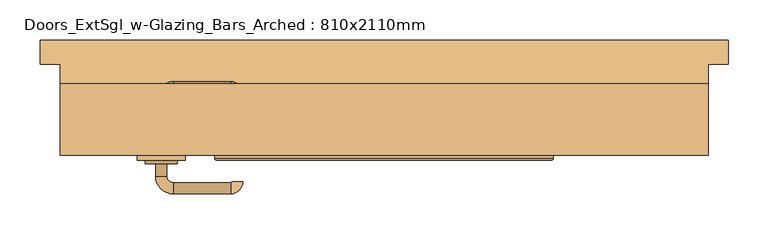
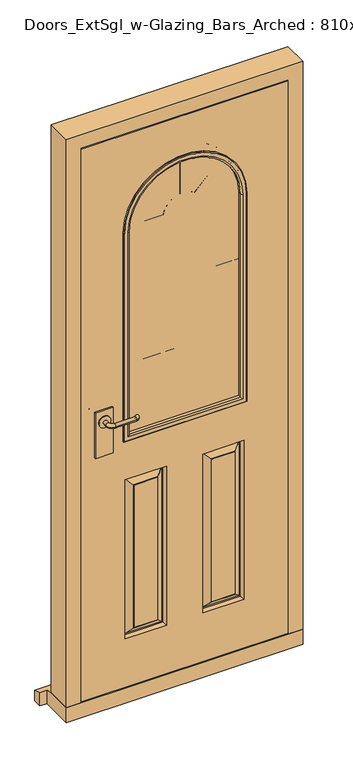
"""IFC4 building model written with IfcOpenShell, lengths in millimetres: door geometry, Doors_ExtSgl_w-Glazing_Bars_Arched : 810x2110mm."""

from ifc_helpers import new_model, si_unit, point, frame, frame_2d, origin, place, context, project, spatial, polyline, circle_curve, ellipse_curve, trimmed, segment, composite_curve, outline, extrude, faceted_brep, source, transform, mapped, element, save
from ifc_brep_helpers import plane_surface, cylinder_surface, revolved_surface, advanced_brep


def doors_extsgl_w_glazing_bars_arched_810x2110mm_57ea6d9e(model_context):
    return source(origin(), model_context, "Body", "SolidModel", [
        extrude(outline(composite_curve([segment(trimmed(circle_curve(frame_2d((1050.0, -278.5)), 20.0), [point((1050.0, -298.5))], [point((1050.0, -258.5))], False, "CARTESIAN"), True, "CONTINUOUS"), segment(trimmed(circle_curve(frame_2d((1050.0, -278.5)), 20.0), [point((1050.0, -258.5))], [point((1050.0, -298.5))], False, "CARTESIAN"), True, "CONTINUOUS")], self_intersect=False)), frame((0.0, -22.9929895, 0.0), z_axis=(0.0, 1.0, 0.0), x_axis=(0.0, 0.0, 1.0)), (0.0, 0.0, 1.0), 4.5929895),
        advanced_brep(
        [(-271.5, -22.9929895, 1050.0), (-285.5, -22.9929895, 1050.0), (-285.5, -38.4, 1050.0), (-271.5, -38.4, 1050.0), (-263.5, -60.4, 1050.0), (-263.5, -46.4, 1050.0), (-191.5, -60.4, 1050.0), (-191.5, -46.4, 1050.0), (-190.5, -45.4, 1050.0), (-176.5, -45.4, 1050.0)],
        [
            (0, 1, circle_curve(frame((-278.5, -22.9929895, 1050.0), z_axis=(0.0, 1.0, 0.0), x_axis=(-1.0, 0.0, 0.0)), 7.0)),
            (1, 0, circle_curve(frame((-278.5, -22.9929895, 1050.0), z_axis=(0.0, 1.0, 0.0), x_axis=(-1.0, 0.0, 0.0)), 7.0)),
            (1, 2),
            (2, 3, circle_curve(frame((-278.5, -38.4, 1050.0), z_axis=(0.0, 1.0, 0.0), x_axis=(-1.0, 0.0, 0.0)), 7.0)),
            (3, 0),
            (3, 2, circle_curve(frame((-278.5, -38.4, 1050.0), z_axis=(0.0, 1.0, 0.0), x_axis=(-1.0, 0.0, 0.0)), 7.0)),
            (4, 5, circle_curve(frame((-263.5, -53.4, 1050.0), z_axis=(-1.0, 0.0, 0.0), x_axis=(0.0, -1.0, 0.0)), 7.0)),
            (5, 3, circle_curve(frame((-263.5, -38.4, 1050.0), z_axis=(0.0, 0.0, -1.0), x_axis=(-1.0, 0.0, 0.0)), 8.0)),
            (2, 4, circle_curve(frame((-263.5, -38.4, 1050.0), z_axis=(0.0, 0.0, 1.0), x_axis=(-1.0, 0.0, 0.0)), 22.0)),
            (5, 4, circle_curve(frame((-263.5, -53.4, 1050.0), z_axis=(-1.0, 0.0, 0.0), x_axis=(0.0, -1.0, 0.0)), 7.0)),
            (4, 6),
            (6, 7, circle_curve(frame((-191.5, -53.4, 1050.0), z_axis=(-1.0, 0.0, 0.0), x_axis=(0.0, -1.0, 0.0)), 7.0)),
            (7, 5),
            (7, 6, circle_curve(frame((-191.5, -53.4, 1050.0), z_axis=(-1.0, 0.0, 0.0), x_axis=(0.0, -1.0, 0.0)), 7.0)),
            (8, 9, circle_curve(frame((-183.5, -45.4, 1050.0), z_axis=(0.0, 1.0, 0.0), x_axis=(1.0, 0.0, 0.0)), 7.0)),
            (9, 8, circle_curve(frame((-183.5, -45.4, 1050.0), z_axis=(0.0, 1.0, 0.0), x_axis=(1.0, 0.0, 0.0)), 7.0)),
            (8, 7, circle_curve(frame((-191.5, -45.4, 1050.0), z_axis=(0.0, 0.0, -1.0), x_axis=(0.0, -1.0, 0.0)), 1.0)),
            (6, 9, circle_curve(frame((-191.5, -45.4, 1050.0), z_axis=(0.0, 0.0, 1.0), x_axis=(0.0, -1.0, 0.0)), 15.0)),
        ],
        [
            plane_surface(frame((-278.5, -22.9929895, 1050.0), z_axis=(0.0, 1.0, 0.0), x_axis=(0.0, 0.0, 1.0))),
            cylinder_surface(frame((-278.5, -22.9929895, 1050.0), z_axis=(0.0, 1.0, 0.0), x_axis=(-1.0, 0.0, 0.0)), 7.0),
            revolved_surface(trimmed(ellipse_curve(frame((-278.5, -38.4, 1050.0), z_axis=(0.0, -1.0, 0.0), x_axis=(-1.0, 0.0, 0.0)), 7.0, 7.0), [point((-271.5, -38.4, 1050.0))], [point((-285.5, -38.4, 1050.0))], True, "CARTESIAN"), (-263.5, -38.4, 1050.0), (0.0, 0.0, -1.0)),
            revolved_surface(trimmed(ellipse_curve(frame((-278.5, -38.4, 1050.0), z_axis=(0.0, -1.0, 0.0), x_axis=(-1.0, 0.0, 0.0)), 7.0, 7.0), [point((-285.5, -38.4, 1050.0))], [point((-271.5, -38.4, 1050.0))], True, "CARTESIAN"), (-263.5, -38.4, 1050.0), (0.0, 0.0, -1.0)),
            cylinder_surface(frame((-263.5, -53.4, 1050.0), z_axis=(-1.0, 0.0, 0.0), x_axis=(0.0, -1.0, 0.0)), 7.0),
            plane_surface(frame((-183.5, -45.4, 1050.0), z_axis=(0.0, 1.0, 0.0), x_axis=(0.0, 0.0, 1.0))),
            revolved_surface(trimmed(ellipse_curve(frame((-191.5, -53.4, 1050.0), z_axis=(1.0, 0.0, 0.0), x_axis=(0.0, -1.0, 0.0)), 7.0, 7.0), [point((-191.5, -46.4, 1050.0))], [point((-191.5, -60.4, 1050.0))], True, "CARTESIAN"), (-191.5, -45.4, 1050.0), (0.0, 0.0, -1.0)),
            revolved_surface(trimmed(ellipse_curve(frame((-191.5, -53.4, 1050.0), z_axis=(1.0, 0.0, 0.0), x_axis=(0.0, -1.0, 0.0)), 7.0, 7.0), [point((-191.5, -60.4, 1050.0))], [point((-191.5, -46.4, 1050.0))], True, "CARTESIAN"), (-191.5, -45.4, 1050.0), (0.0, 0.0, -1.0)),
        ],
        [
            (0, [[1, 2]]),
            (1, [[3, 4, 5, -2]]),
            (1, [[-5, 6, -3, -1]]),
            (2, [[7, 8, -4, 9]]),
            (3, [[10, -9, -6, -8]]),
            (4, [[11, 12, 13, -7]]),
            (4, [[-13, 14, -11, -10]]),
            (5, [[15, 16]]),
            (6, [[-15, 17, -12, 18]]),
            (7, [[-16, -18, -14, -17]]),
        ],
    ),
        extrude(outline(polyline([(-248.5, -12.4), (-248.5, -18.4), (-308.5, -18.4), (-308.5, -12.4), (-248.5, -12.4)])), frame((0.0, 0.0, 925.0), z_axis=(0.0, 0.0, 1.0), x_axis=(1.0, 0.0, 0.0)), (0.0, 0.0, 1.0), 165.0),
        extrude(outline(composite_curve([segment(trimmed(circle_curve(frame_2d((1050.0, -278.5)), 20.0), [point((1050.0, -298.5))], [point((1050.0, -258.5))], False, "CARTESIAN"), True, "CONTINUOUS"), segment(trimmed(circle_curve(frame_2d((1050.0, -278.5)), 20.0), [point((1050.0, -258.5))], [point((1050.0, -298.5))], False, "CARTESIAN"), True, "CONTINUOUS")], self_intersect=False)), frame((0.0, 37.6, 0.0), z_axis=(0.0, 1.0, 0.0), x_axis=(0.0, 0.0, 1.0)), (0.0, 0.0, 1.0), 4.5929895),
        advanced_brep(
        [(-271.5, 42.1929895, 1050.0), (-285.5, 42.1929895, 1050.0), (-271.5, 57.6, 1050.0), (-285.5, 57.6, 1050.0), (-263.5, 79.6, 1050.0), (-263.5, 65.6, 1050.0), (-191.5, 65.6, 1050.0), (-191.5, 79.6, 1050.0), (-190.5, 64.6, 1050.0), (-176.5, 64.6, 1050.0)],
        [
            (0, 1, circle_curve(frame((-278.5, 42.1929895, 1050.0), z_axis=(0.0, -1.0, 0.0), x_axis=(-1.0, 0.0, 0.0)), 7.0)),
            (1, 0, circle_curve(frame((-278.5, 42.1929895, 1050.0), z_axis=(0.0, -1.0, 0.0), x_axis=(-1.0, 0.0, 0.0)), 7.0)),
            (0, 2),
            (2, 3, circle_curve(frame((-278.5, 57.6, 1050.0), z_axis=(0.0, -1.0, 0.0), x_axis=(-1.0, 0.0, 0.0)), 7.0)),
            (3, 1),
            (3, 2, circle_curve(frame((-278.5, 57.6, 1050.0), z_axis=(0.0, -1.0, 0.0), x_axis=(-1.0, 0.0, 0.0)), 7.0)),
            (4, 3, circle_curve(frame((-263.5, 57.6, 1050.0), z_axis=(0.0, 0.0, 1.0), x_axis=(-1.0, 0.0, 0.0)), 22.0)),
            (2, 5, circle_curve(frame((-263.5, 57.6, 1050.0), z_axis=(0.0, 0.0, -1.0), x_axis=(-1.0, 0.0, 0.0)), 8.0)),
            (5, 4, circle_curve(frame((-263.5, 72.6, 1050.0), z_axis=(-1.0, 0.0, 0.0), x_axis=(0.0, 1.0, 0.0)), 7.0)),
            (4, 5, circle_curve(frame((-263.5, 72.6, 1050.0), z_axis=(-1.0, 0.0, 0.0), x_axis=(0.0, 1.0, 0.0)), 7.0)),
            (5, 6),
            (6, 7, circle_curve(frame((-191.5, 72.6, 1050.0), z_axis=(-1.0, 0.0, 0.0), x_axis=(0.0, 1.0, 0.0)), 7.0)),
            (7, 4),
            (7, 6, circle_curve(frame((-191.5, 72.6, 1050.0), z_axis=(-1.0, 0.0, 0.0), x_axis=(0.0, 1.0, 0.0)), 7.0)),
            (8, 9, circle_curve(frame((-183.5, 64.6, 1050.0), z_axis=(0.0, -1.0, 0.0), x_axis=(1.0, 0.0, 0.0)), 7.0)),
            (9, 8, circle_curve(frame((-183.5, 64.6, 1050.0), z_axis=(0.0, -1.0, 0.0), x_axis=(1.0, 0.0, 0.0)), 7.0)),
            (9, 7, circle_curve(frame((-191.5, 64.6, 1050.0), z_axis=(0.0, 0.0, 1.0), x_axis=(0.0, 1.0, 0.0)), 15.0)),
            (6, 8, circle_curve(frame((-191.5, 64.6, 1050.0), z_axis=(0.0, 0.0, -1.0), x_axis=(0.0, 1.0, 0.0)), 1.0)),
        ],
        [
            plane_surface(frame((-278.5, 42.1929895, 1050.0), z_axis=(0.0, -1.0, 0.0), x_axis=(0.0, 0.0, 1.0))),
            cylinder_surface(frame((-278.5, 42.1929895, 1050.0), z_axis=(0.0, -1.0, 0.0), x_axis=(-1.0, 0.0, 0.0)), 7.0),
            revolved_surface(trimmed(ellipse_curve(frame((-278.5, 57.6, 1050.0), z_axis=(0.0, -1.0, 0.0), x_axis=(-1.0, 0.0, 0.0)), 7.0, 7.0), [point((-271.5, 57.6, 1050.0))], [point((-285.5, 57.6, 1050.0))], True, "CARTESIAN"), (-263.5, 57.6, 1050.0), (0.0, 0.0, -1.0)),
            revolved_surface(trimmed(ellipse_curve(frame((-278.5, 57.6, 1050.0), z_axis=(0.0, -1.0, 0.0), x_axis=(-1.0, 0.0, 0.0)), 7.0, 7.0), [point((-285.5, 57.6, 1050.0))], [point((-271.5, 57.6, 1050.0))], True, "CARTESIAN"), (-263.5, 57.6, 1050.0), (0.0, 0.0, -1.0)),
            cylinder_surface(frame((-263.5, 72.6, 1050.0), z_axis=(-1.0, 0.0, 0.0), x_axis=(0.0, 1.0, 0.0)), 7.0),
            plane_surface(frame((-183.5, 64.6, 1050.0), z_axis=(0.0, -1.0, 0.0), x_axis=(0.0, 0.0, 1.0))),
            revolved_surface(trimmed(ellipse_curve(frame((-191.5, 72.6, 1050.0), z_axis=(-1.0, 0.0, 0.0), x_axis=(0.0, 1.0, 0.0)), 7.0, 7.0), [point((-191.5, 65.6, 1050.0))], [point((-191.5, 79.6, 1050.0))], True, "CARTESIAN"), (-191.5, 64.6, 1050.0), (0.0, 0.0, -1.0)),
            revolved_surface(trimmed(ellipse_curve(frame((-191.5, 72.6, 1050.0), z_axis=(-1.0, 0.0, 0.0), x_axis=(0.0, 1.0, 0.0)), 7.0, 7.0), [point((-191.5, 79.6, 1050.0))], [point((-191.5, 65.6, 1050.0))], True, "CARTESIAN"), (-191.5, 64.6, 1050.0), (0.0, 0.0, -1.0)),
        ],
        [
            (0, [[1, 2]]),
            (1, [[-1, 3, 4, 5]]),
            (1, [[-2, -5, 6, -3]]),
            (2, [[7, -4, 8, 9]]),
            (3, [[-8, -6, -7, 10]]),
            (4, [[-9, 11, 12, 13]]),
            (4, [[-10, -13, 14, -11]]),
            (5, [[15, 16]]),
            (6, [[17, -12, 18, -16]]),
            (7, [[-18, -14, -17, -15]]),
        ],
    ),
        extrude(outline(polyline([(-248.5, 31.6), (-308.5, 31.6), (-308.5, 37.6), (-248.5, 37.6), (-248.5, 31.6)])), frame((0.0, 0.0, 925.0), z_axis=(0.0, 0.0, 1.0), x_axis=(1.0, 0.0, 0.0)), (0.0, 0.0, 1.0), 165.0),
        faceted_brep([(334.5, 76.6, 54.5), (405.0, 76.6, 54.5), (405.0, -12.4, 54.5), (356.5, -12.4, 54.5), (356.5, 34.6, 54.5), (334.5, 34.6, 54.5), (334.5, 76.6, 2039.5), (-334.5, 76.6, 2039.5), (-334.5, 76.6, 54.5), (-405.0, 76.6, 54.5), (-405.0, 76.6, 2110.0), (405.0, 76.6, 2110.0), (405.0, -12.4, 2110.0), (-405.0, -12.4, 2110.0), (-405.0, -12.4, 54.5), (-356.5, -12.4, 54.5), (-356.5, -12.4, 2061.5), (356.5, -12.4, 2061.5), (356.5, 34.6, 2061.5), (-356.5, 34.6, 2061.5), (-356.5, 34.6, 54.5), (-334.5, 34.6, 54.5), (-334.5, 34.6, 2039.5), (334.5, 34.6, 2039.5)], [[[0, 1, 2, 3, 4, 5]], [[1, 0, 6, 7, 8, 9, 10, 11]], [[2, 1, 11, 12]], [[3, 2, 12, 13, 14, 15, 16, 17]], [[4, 3, 17, 18]], [[5, 4, 18, 19, 20, 21, 22, 23]], [[0, 5, 23, 6]], [[8, 7, 22, 21]], [[9, 8, 21, 20, 15, 14]], [[10, 9, 14, 13]], [[16, 15, 20, 19]], [[11, 10, 13, 12]], [[17, 16, 19, 18]], [[7, 6, 23, 22]]]),
        advanced_brep(
        [(353.5, -12.4, 58.5), (353.5, -12.4, 2058.5), (-354.4250294, -12.4, 2058.5), (-354.4250294, -12.4, 58.5), (-203.5, -12.4, 958.5), (-203.5, -12.4, 1705.0), (203.5, -12.4, 1705.0), (203.5, -12.4, 958.5), (-62.5, -12.4, 808.5), (-62.5, -12.4, 233.5), (-203.5, -12.4, 233.5), (-203.5, -12.4, 808.5), (203.5, -12.4, 808.5), (203.5, -12.4, 233.5), (62.5, -12.4, 233.5), (62.5, -12.4, 808.5), (-92.5, -12.4, 263.5), (-92.5, -12.4, 778.5), (-173.5, -12.4, 778.5), (-173.5, -12.4, 263.5), (173.5, -12.4, 263.5), (173.5, -12.4, 778.5), (92.5, -12.4, 778.5), (92.5, -12.4, 263.5), (353.5, 31.6, 58.5), (-354.4250294, 31.6, 58.5), (-354.4250294, 31.6, 2058.5), (353.5, 31.6, 2058.5), (-203.5, 31.6, 958.5), (203.5, 31.6, 958.5), (203.5, 31.6, 1705.0), (-203.5, 31.6, 1705.0), (62.5, 31.6, 808.5), (62.5, 31.6, 233.5), (203.5, 31.6, 233.5), (203.5, 31.6, 808.5), (-203.5, 31.6, 808.5), (-203.5, 31.6, 233.5), (-62.5, 31.6, 233.5), (-62.5, 31.6, 808.5), (92.5, 31.6, 263.5), (92.5, 31.6, 778.5), (173.5, 31.6, 778.5), (173.5, 31.6, 263.5), (-173.5, 31.6, 263.5), (-173.5, 31.6, 778.5), (-92.5, 31.6, 778.5), (-92.5, 31.6, 263.5), (65.5, 16.6, 805.5), (65.5, 16.6, 236.5), (90.5, 30.6, 780.5), (90.5, 30.6, 261.5), (70.5, 16.6, 241.5), (70.5, 16.6, 800.5), (92.5, 30.6, 263.5), (92.5, 30.6, 778.5), (200.5, 16.6, 236.5), (175.5, 30.6, 261.5), (195.5, 16.6, 241.5), (173.5, 30.6, 263.5), (200.5, 16.6, 805.5), (175.5, 30.6, 780.5), (195.5, 16.6, 800.5), (173.5, 30.6, 778.5), (-200.5, 16.6, 805.5), (-200.5, 16.6, 236.5), (-175.5, 30.6, 780.5), (-175.5, 30.6, 261.5), (-195.5, 16.6, 241.5), (-195.5, 16.6, 800.5), (-173.5, 30.6, 263.5), (-173.5, 30.6, 778.5), (-65.5, 16.6, 236.5), (-90.5, 30.6, 261.5), (-70.5, 16.6, 241.5), (-92.5, 30.6, 263.5), (-65.5, 16.6, 805.5), (-90.5, 30.6, 780.5), (-70.5, 16.6, 800.5), (-92.5, 30.6, 778.5), (-92.5, -11.4, 263.5), (-92.5, -11.4, 778.5), (-70.5, 2.6, 241.5), (-70.5, 2.6, 800.5), (-90.5, -11.4, 780.5), (-90.5, -11.4, 261.5), (-65.5, 2.6, 805.5), (-65.5, 2.6, 236.5), (-173.5, -11.4, 778.5), (-195.5, 2.6, 800.5), (-175.5, -11.4, 780.5), (-200.5, 2.6, 805.5), (-173.5, -11.4, 263.5), (-195.5, 2.6, 241.5), (-175.5, -11.4, 261.5), (-200.5, 2.6, 236.5), (200.5, 2.6, 805.5), (200.5, 2.6, 236.5), (175.5, -11.4, 780.5), (175.5, -11.4, 261.5), (195.5, 2.6, 241.5), (195.5, 2.6, 800.5), (173.5, -11.4, 263.5), (173.5, -11.4, 778.5), (65.5, 2.6, 236.5), (90.5, -11.4, 261.5), (70.5, 2.6, 241.5), (92.5, -11.4, 263.5), (65.5, 2.6, 805.5), (90.5, -11.4, 780.5), (70.5, 2.6, 800.5), (92.5, -11.4, 778.5)],
        [
            (0, 1),
            (1, 2),
            (2, 3),
            (3, 0),
            (4, 5),
            (5, 6, circle_curve(frame((0.0, -12.4, 1705.0), z_axis=(0.0, 1.0, 0.0), x_axis=(1.0, 0.0, 0.0)), 203.5)),
            (6, 7),
            (7, 4),
            (8, 9),
            (9, 10),
            (10, 11),
            (11, 8),
            (12, 13),
            (13, 14),
            (14, 15),
            (15, 12),
            (16, 17),
            (17, 18),
            (18, 19),
            (19, 16),
            (20, 21),
            (21, 22),
            (22, 23),
            (23, 20),
            (24, 25),
            (25, 26),
            (26, 27),
            (27, 24),
            (28, 29),
            (29, 30),
            (30, 31, circle_curve(frame((0.0, 31.6, 1705.0), z_axis=(0.0, -1.0, 0.0), x_axis=(1.0, 0.0, 0.0)), 203.5)),
            (31, 28),
            (32, 33),
            (33, 34),
            (34, 35),
            (35, 32),
            (36, 37),
            (37, 38),
            (38, 39),
            (39, 36),
            (40, 41),
            (41, 42),
            (42, 43),
            (43, 40),
            (44, 45),
            (45, 46),
            (46, 47),
            (47, 44),
            (0, 24),
            (27, 1),
            (26, 2),
            (25, 3),
            (4, 28),
            (31, 5),
            (30, 6),
            (29, 7),
            (48, 49),
            (49, 33),
            (32, 48),
            (50, 51),
            (51, 52),
            (52, 53),
            (53, 50),
            (40, 54),
            (54, 55),
            (55, 41),
            (49, 56),
            (56, 34),
            (51, 57),
            (57, 58),
            (58, 52),
            (43, 59),
            (59, 54),
            (56, 60),
            (60, 35),
            (57, 61),
            (61, 62),
            (62, 58),
            (42, 63),
            (63, 59),
            (60, 48),
            (62, 53),
            (61, 50),
            (63, 55),
            (64, 65),
            (65, 37),
            (36, 64),
            (66, 67),
            (67, 68),
            (68, 69),
            (69, 66),
            (44, 70),
            (70, 71),
            (71, 45),
            (65, 72),
            (72, 38),
            (67, 73),
            (73, 74),
            (74, 68),
            (47, 75),
            (75, 70),
            (72, 76),
            (76, 39),
            (73, 77),
            (77, 78),
            (78, 74),
            (46, 79),
            (79, 75),
            (76, 64),
            (78, 69),
            (77, 66),
            (79, 71),
            (80, 81),
            (81, 17),
            (16, 80),
            (82, 83),
            (83, 84),
            (84, 85),
            (85, 82),
            (8, 86),
            (86, 87),
            (87, 9),
            (81, 88),
            (88, 18),
            (83, 89),
            (89, 90),
            (90, 84),
            (11, 91),
            (91, 86),
            (88, 92),
            (92, 19),
            (89, 93),
            (93, 94),
            (94, 90),
            (10, 95),
            (95, 91),
            (92, 80),
            (94, 85),
            (93, 82),
            (95, 87),
            (96, 97),
            (97, 13),
            (12, 96),
            (98, 99),
            (99, 100),
            (100, 101),
            (101, 98),
            (20, 102),
            (102, 103),
            (103, 21),
            (97, 104),
            (104, 14),
            (99, 105),
            (105, 106),
            (106, 100),
            (23, 107),
            (107, 102),
            (104, 108),
            (108, 15),
            (105, 109),
            (109, 110),
            (110, 106),
            (22, 111),
            (111, 107),
            (108, 96),
            (110, 101),
            (109, 98),
            (111, 103),
        ],
        [
            plane_surface(frame((353.5, -12.4, 58.5), z_axis=(0.0, -1.0, 0.0), x_axis=(0.0, 0.0, 1.0))),
            plane_surface(frame((353.5, 31.6, 58.5), z_axis=(0.0, 1.0, 0.0), x_axis=(0.0, 0.0, -1.0))),
            plane_surface(frame((353.5, -12.4, 58.5), z_axis=(1.0, 0.0, 0.0), x_axis=(0.0, 1.0, 0.0))),
            plane_surface(frame((353.5, -12.4, 2058.5), z_axis=(0.0, 0.0, 1.0), x_axis=(0.0, 1.0, 0.0))),
            plane_surface(frame((-354.4250294, -12.4, 2058.5), z_axis=(-1.0, 0.0, 0.0), x_axis=(0.0, 1.0, 0.0))),
            plane_surface(frame((-354.4250294, -12.4, 58.5), z_axis=(0.0, 0.0, -1.0), x_axis=(0.0, 1.0, 0.0))),
            plane_surface(frame((-203.5, -12.4, 958.5), z_axis=(1.0, 0.0, 0.0), x_axis=(0.0, 1.0, 0.0))),
            revolved_surface(polyline([(203.5, 31.6, 1705.0), (203.5, -12.4, 1705.0)]), (0.0, -12.4, 1705.0), (0.0, 1.0, 0.0)),
            plane_surface(frame((203.5, -12.4, 1705.0), z_axis=(-1.0, 0.0, 0.0), x_axis=(0.0, 1.0, 0.0))),
            plane_surface(frame((203.5, -12.4, 958.5), z_axis=(0.0, 0.0, 1.0), x_axis=(0.0, 1.0, 0.0))),
            plane_surface(frame((62.5, 31.6, 808.5), z_axis=(0.9805806756909202, 0.19611613513818407, 0.0), x_axis=(0.0, 0.0, -1.0))),
            plane_surface(frame((70.5, 16.6, 800.5), z_axis=(-0.5734623443633278, 0.8192319205190408, 0.0), x_axis=(0.0, 0.0, -1.0))),
            plane_surface(frame((92.5, 30.6, 778.5), z_axis=(-1.0, 0.0, 0.0), x_axis=(0.0, 0.0, -1.0))),
            plane_surface(frame((62.5, 31.6, 233.5), z_axis=(0.0, 0.19611613513818718, 0.9805806756909196), x_axis=(1.0, 0.0, 0.0))),
            plane_surface(frame((70.5, 16.6, 241.5), z_axis=(0.0, 0.8192319205190389, -0.5734623443633305), x_axis=(1.0, 0.0, 0.0))),
            plane_surface(frame((92.5, 30.6, 263.5), z_axis=(0.0, 0.0, -1.0), x_axis=(1.0, 0.0, 0.0))),
            plane_surface(frame((203.5, 31.6, 233.5), z_axis=(-0.9805806756909189, 0.19611613513819035, 0.0), x_axis=(0.0, 0.0, 1.0))),
            plane_surface(frame((195.5, 16.6, 241.5), z_axis=(0.5734623443633332, 0.819231920519037, 0.0), x_axis=(0.0, 0.0, 1.0))),
            plane_surface(frame((173.5, 30.6, 263.5), z_axis=(1.0, 0.0, 0.0), x_axis=(0.0, 0.0, 1.0))),
            plane_surface(frame((203.5, 31.6, 808.5), z_axis=(0.0, 0.19611613513818718, -0.9805806756909196), x_axis=(-1.0, 0.0, 0.0))),
            plane_surface(frame((200.5, 16.6, 805.5), z_axis=(0.0, 1.0, 0.0), x_axis=(-1.0, 0.0, 0.0))),
            plane_surface(frame((195.5, 16.6, 800.5), z_axis=(0.0, 0.8192319205190389, 0.5734623443633305), x_axis=(-1.0, 0.0, 0.0))),
            plane_surface(frame((175.5, 30.6, 780.5), z_axis=(0.0, 1.0, 0.0), x_axis=(-1.0, 0.0, 0.0))),
            plane_surface(frame((173.5, 30.6, 778.5), z_axis=(0.0, 0.0, 1.0), x_axis=(-1.0, 0.0, 0.0))),
            plane_surface(frame((-203.5, 31.6, 808.5), z_axis=(0.9805806756909202, 0.19611613513818407, 0.0), x_axis=(0.0, 0.0, -1.0))),
            plane_surface(frame((-195.5, 16.6, 800.5), z_axis=(-0.5734623443633278, 0.8192319205190408, 0.0), x_axis=(0.0, 0.0, -1.0))),
            plane_surface(frame((-173.5, 30.6, 778.5), z_axis=(-1.0, 0.0, 0.0), x_axis=(0.0, 0.0, -1.0))),
            plane_surface(frame((-203.5, 31.6, 233.5), z_axis=(0.0, 0.19611613513818724, 0.9805806756909196), x_axis=(1.0, 0.0, 0.0))),
            plane_surface(frame((-195.5, 16.6, 241.5), z_axis=(0.0, 0.819231920519039, -0.5734623443633305), x_axis=(1.0, 0.0, 0.0))),
            plane_surface(frame((-173.5, 30.6, 263.5), z_axis=(0.0, 0.0, -1.0), x_axis=(1.0, 0.0, 0.0))),
            plane_surface(frame((-62.5, 31.6, 233.5), z_axis=(-0.9805806756909189, 0.1961161351381904, 0.0), x_axis=(0.0, 0.0, 1.0))),
            plane_surface(frame((-70.5, 16.6, 241.5), z_axis=(0.5734623443633332, 0.8192319205190371, 0.0), x_axis=(0.0, 0.0, 1.0))),
            plane_surface(frame((-92.5, 30.6, 263.5), z_axis=(1.0, 0.0, 0.0), x_axis=(0.0, 0.0, 1.0))),
            plane_surface(frame((-62.5, 31.6, 808.5), z_axis=(0.0, 0.19611613513818724, -0.9805806756909196), x_axis=(-1.0, 0.0, 0.0))),
            plane_surface(frame((-65.5, 16.6, 805.5), z_axis=(0.0, 1.0, 0.0), x_axis=(-1.0, 0.0, 0.0))),
            plane_surface(frame((-70.5, 16.6, 800.5), z_axis=(0.0, 0.819231920519039, 0.5734623443633305), x_axis=(-1.0, 0.0, 0.0))),
            plane_surface(frame((-90.5, 30.6, 780.5), z_axis=(0.0, 1.0, 0.0), x_axis=(-1.0, 0.0, 0.0))),
            plane_surface(frame((-92.5, 30.6, 778.5), z_axis=(0.0, 0.0, 1.0), x_axis=(-1.0, 0.0, 0.0))),
            plane_surface(frame((-92.5, -12.4, 263.5), z_axis=(1.0, 0.0, 0.0), x_axis=(0.0, 0.0, 1.0))),
            plane_surface(frame((-90.5, -11.4, 261.5), z_axis=(0.5734623443633226, -0.8192319205190445, 0.0), x_axis=(0.0, 0.0, 1.0))),
            plane_surface(frame((-65.5, 2.6, 236.5), z_axis=(-0.9805806756909214, -0.1961161351381777, 0.0), x_axis=(0.0, 0.0, 1.0))),
            plane_surface(frame((-92.5, -12.4, 778.5), z_axis=(0.0, 0.0, 1.0), x_axis=(-1.0, 0.0, 0.0))),
            plane_surface(frame((-90.5, -11.4, 780.5), z_axis=(0.0, -0.8192319205190427, 0.5734623443633253), x_axis=(-1.0, 0.0, 0.0))),
            plane_surface(frame((-65.5, 2.6, 805.5), z_axis=(0.0, -0.19611613513818085, -0.9805806756909208), x_axis=(-1.0, 0.0, 0.0))),
            plane_surface(frame((-173.5, -12.4, 778.5), z_axis=(-1.0, 0.0, 0.0), x_axis=(0.0, 0.0, -1.0))),
            plane_surface(frame((-175.5, -11.4, 780.5), z_axis=(-0.5734623443633281, -0.8192319205190407, 0.0), x_axis=(0.0, 0.0, -1.0))),
            plane_surface(frame((-200.5, 2.6, 805.5), z_axis=(0.9805806756909202, -0.196116135138184, 0.0), x_axis=(0.0, 0.0, -1.0))),
            plane_surface(frame((-173.5, -12.4, 263.5), z_axis=(0.0, 0.0, -1.0), x_axis=(1.0, 0.0, 0.0))),
            plane_surface(frame((-173.5, -11.4, 263.5), z_axis=(0.0, -1.0, 0.0), x_axis=(1.0, 0.0, 0.0))),
            plane_surface(frame((-175.5, -11.4, 261.5), z_axis=(0.0, -0.8192319205190426, -0.5734623443633253), x_axis=(1.0, 0.0, 0.0))),
            plane_surface(frame((-195.5, 2.6, 241.5), z_axis=(0.0, -1.0, 0.0), x_axis=(1.0, 0.0, 0.0))),
            plane_surface(frame((-200.5, 2.6, 236.5), z_axis=(0.0, -0.19611613513818088, 0.9805806756909209), x_axis=(1.0, 0.0, 0.0))),
            plane_surface(frame((203.5, -12.4, 808.5), z_axis=(-0.9805806756909202, -0.19611613513818407, 0.0), x_axis=(0.0, 0.0, -1.0))),
            plane_surface(frame((195.5, 2.6, 800.5), z_axis=(0.5734623443633278, -0.8192319205190408, 0.0), x_axis=(0.0, 0.0, -1.0))),
            plane_surface(frame((173.5, -11.4, 778.5), z_axis=(1.0, 0.0, 0.0), x_axis=(0.0, 0.0, -1.0))),
            plane_surface(frame((203.5, -12.4, 233.5), z_axis=(0.0, -0.19611613513818724, 0.9805806756909196), x_axis=(-1.0, 0.0, 0.0))),
            plane_surface(frame((195.5, 2.6, 241.5), z_axis=(0.0, -0.819231920519039, -0.5734623443633305), x_axis=(-1.0, 0.0, 0.0))),
            plane_surface(frame((173.5, -11.4, 263.5), z_axis=(0.0, 0.0, -1.0), x_axis=(-1.0, 0.0, 0.0))),
            plane_surface(frame((62.5, -12.4, 233.5), z_axis=(0.9805806756909189, -0.19611613513819046, 0.0), x_axis=(0.0, 0.0, 1.0))),
            plane_surface(frame((70.5, 2.6, 241.5), z_axis=(-0.5734623443633331, -0.8192319205190371, 0.0), x_axis=(0.0, 0.0, 1.0))),
            plane_surface(frame((92.5, -11.4, 263.5), z_axis=(-1.0, 0.0, 0.0), x_axis=(0.0, 0.0, 1.0))),
            plane_surface(frame((62.5, -12.4, 808.5), z_axis=(0.0, -0.19611613513818724, -0.9805806756909196), x_axis=(1.0, 0.0, 0.0))),
            plane_surface(frame((65.5, 2.6, 805.5), z_axis=(0.0, -1.0, 0.0), x_axis=(1.0, 0.0, 0.0))),
            plane_surface(frame((70.5, 2.6, 800.5), z_axis=(0.0, -0.819231920519039, 0.5734623443633305), x_axis=(1.0, 0.0, 0.0))),
            plane_surface(frame((90.5, -11.4, 780.5), z_axis=(0.0, -1.0, 0.0), x_axis=(1.0, 0.0, 0.0))),
            plane_surface(frame((92.5, -11.4, 778.5), z_axis=(0.0, 0.0, 1.0), x_axis=(1.0, 0.0, 0.0))),
        ],
        [
            (0, [[1, 2, 3, 4], [5, 6, 7, 8], [9, 10, 11, 12], [13, 14, 15, 16]]),
            (0, [[17, 18, 19, 20]]),
            (0, [[21, 22, 23, 24]]),
            (1, [[25, 26, 27, 28], [29, 30, 31, 32], [33, 34, 35, 36], [37, 38, 39, 40]]),
            (1, [[41, 42, 43, 44]]),
            (1, [[45, 46, 47, 48]]),
            (2, [[-1, 49, -28, 50]]),
            (3, [[-2, -50, -27, 51]]),
            (4, [[-3, -51, -26, 52]]),
            (5, [[-4, -52, -25, -49]]),
            (6, [[-5, 53, -32, 54]]),
            (7, [[-6, -54, -31, 55]]),
            (8, [[-7, -55, -30, 56]]),
            (9, [[-8, -56, -29, -53]]),
            (10, [[57, 58, -33, 59]]),
            (11, [[60, 61, 62, 63]]),
            (12, [[64, 65, 66, -41]]),
            (13, [[-58, 67, 68, -34]]),
            (14, [[-61, 69, 70, 71]]),
            (15, [[-64, -44, 72, 73]]),
            (16, [[-68, 74, 75, -35]]),
            (17, [[-70, 76, 77, 78]]),
            (18, [[-72, -43, 79, 80]]),
            (19, [[-59, -36, -75, 81]]),
            (20, [[-57, -81, -74, -67], [-62, -71, -78, 82]]),
            (21, [[-63, -82, -77, 83]]),
            (22, [[-60, -83, -76, -69], [-65, -73, -80, 84]]),
            (23, [[-66, -84, -79, -42]]),
            (24, [[85, 86, -37, 87]]),
            (25, [[88, 89, 90, 91]]),
            (26, [[92, 93, 94, -45]]),
            (27, [[-86, 95, 96, -38]]),
            (28, [[-89, 97, 98, 99]]),
            (29, [[-92, -48, 100, 101]]),
            (30, [[-96, 102, 103, -39]]),
            (31, [[-98, 104, 105, 106]]),
            (32, [[-100, -47, 107, 108]]),
            (33, [[-87, -40, -103, 109]]),
            (34, [[-85, -109, -102, -95], [-90, -99, -106, 110]]),
            (35, [[-91, -110, -105, 111]]),
            (36, [[-88, -111, -104, -97], [-93, -101, -108, 112]]),
            (37, [[-94, -112, -107, -46]]),
            (38, [[113, 114, -17, 115]]),
            (39, [[116, 117, 118, 119]]),
            (40, [[120, 121, 122, -9]]),
            (41, [[-114, 123, 124, -18]]),
            (42, [[-117, 125, 126, 127]]),
            (43, [[-120, -12, 128, 129]]),
            (44, [[-124, 130, 131, -19]]),
            (45, [[-126, 132, 133, 134]]),
            (46, [[-128, -11, 135, 136]]),
            (47, [[-115, -20, -131, 137]]),
            (48, [[-118, -127, -134, 138], [-113, -137, -130, -123]]),
            (49, [[-119, -138, -133, 139]]),
            (50, [[-121, -129, -136, 140], [-116, -139, -132, -125]]),
            (51, [[-122, -140, -135, -10]]),
            (52, [[141, 142, -13, 143]]),
            (53, [[144, 145, 146, 147]]),
            (54, [[148, 149, 150, -21]]),
            (55, [[-142, 151, 152, -14]]),
            (56, [[-145, 153, 154, 155]]),
            (57, [[-148, -24, 156, 157]]),
            (58, [[-152, 158, 159, -15]]),
            (59, [[-154, 160, 161, 162]]),
            (60, [[-156, -23, 163, 164]]),
            (61, [[-143, -16, -159, 165]]),
            (62, [[-141, -165, -158, -151], [-146, -155, -162, 166]]),
            (63, [[-147, -166, -161, 167]]),
            (64, [[-144, -167, -160, -153], [-149, -157, -164, 168]]),
            (65, [[-150, -168, -163, -22]]),
        ],
    ),
        faceted_brep([(430.0, 131.6, 0.0), (430.0, 131.6, 38.5947221), (430.0, 101.6, 47.2703282), (430.0, 101.6, 0.0), (-430.0, 131.6, 38.5947221), (-430.0, 131.6, 0.0), (-430.0, 101.6, 0.0), (-430.0, 101.6, 47.2703282), (405.0, 101.6, 0.0), (405.0, -12.4, 0.0), (-405.0, -12.4, 0.0), (-405.0, 101.6, 0.0), (-405.0, 101.6, 47.2703282), (-405.0, 76.6, 54.5), (405.0, 76.6, 54.5), (405.0, 101.6, 47.2703282), (-405.0, -12.4, 54.5), (405.0, -12.4, 54.5)], [[[0, 1, 2, 3]], [[4, 5, 6, 7]], [[5, 0, 3, 8, 9, 10, 11, 6]], [[1, 0, 5, 4]], [[1, 4, 7, 12, 13, 14, 15, 2]], [[13, 16, 17, 14]], [[16, 10, 9, 17]], [[12, 11, 10, 16, 13]], [[11, 12, 7, 6]], [[8, 15, 14, 17, 9]], [[15, 8, 3, 2]]]),
        extrude(outline(composite_curve([segment(polyline([(958.5, -203.5), (958.5, 203.5), (1705.0, 203.5)]), True, "CONTINUOUS"), segment(trimmed(circle_curve(frame_2d((1705.0, 0.0)), 203.5), [point((1705.0, 203.5))], [point((1705.0, -203.5))], False, "CARTESIAN"), True, "CONTINUOUS"), segment(polyline([(1705.0, -203.5), (958.5, -203.5)]), True, "CONTINUOUS")], self_intersect=False)), frame((0.0, -2.4, 0.0), z_axis=(0.0, 1.0, 0.0), x_axis=(0.0, 0.0, 1.0)), (0.0, 0.0, 1.0), 24.0),
        advanced_brep(
        [(-211.5, 35.6, 950.5), (-211.5, 31.6, 950.5), (-211.5, 31.6, 1705.0), (-211.5, 35.6, 1705.0), (-209.5, 37.6, 952.5), (-209.5, 37.6, 1705.0), (-191.5, 32.6, 970.5), (-196.5, 37.6, 965.5), (-196.5, 37.6, 1705.0), (-191.5, 32.6, 1705.0), (-191.5, 21.6, 970.5), (-191.5, 21.6, 1705.0), (-203.5, 31.6, 958.5), (-203.5, 21.6, 958.5), (-203.5, 21.6, 1705.0), (-203.5, 31.6, 1705.0), (211.5, 35.6, 1705.0), (211.5, 31.6, 1705.0), (209.5, 37.6, 1705.0), (209.5, 37.6, 952.5), (196.5, 37.6, 1705.0), (196.5, 37.6, 965.5), (191.5, 32.6, 1705.0), (191.5, 21.6, 1705.0), (203.5, 21.6, 1705.0), (203.5, 21.6, 958.5), (191.5, 21.6, 970.5), (203.5, 31.6, 1705.0), (211.5, 31.6, 950.5), (203.5, 31.6, 958.5), (211.5, 35.6, 950.5), (191.5, 32.6, 970.5)],
        [
            (0, 1),
            (1, 2),
            (2, 3),
            (3, 0),
            (4, 0, ellipse_curve(frame((-209.5, 35.6, 952.5), z_axis=(-0.7071067811865475, 0.0, 0.7071067811865475), x_axis=(-0.7071067811865472, 0.0, -0.7071067811865477)), 2.8284271, 2.0)),
            (3, 5, circle_curve(frame((-209.5, 35.6, 1705.0), z_axis=(0.0, 0.0, -1.0), x_axis=(-1.0, 0.0, 0.0)), 2.0)),
            (5, 4),
            (6, 7, ellipse_curve(frame((-196.5, 32.6, 965.5), z_axis=(-0.7071067811865475, 0.0, 0.7071067811865475), x_axis=(-0.7071067811865472, 0.0, -0.7071067811865477)), 7.0710678, 5.0)),
            (7, 8),
            (8, 9, circle_curve(frame((-196.5, 32.6, 1705.0), z_axis=(0.0, 0.0, -1.0), x_axis=(-1.0, 0.0, 0.0)), 5.0)),
            (9, 6),
            (10, 6),
            (9, 11),
            (11, 10),
            (12, 13),
            (13, 14),
            (14, 15),
            (15, 12),
            (16, 3, circle_curve(frame((0.0, 35.6, 1705.0), z_axis=(0.0, -1.0, 0.0), x_axis=(-1.0, 0.0, 0.0)), 211.5)),
            (2, 17, circle_curve(frame((0.0, 31.6, 1705.0), z_axis=(0.0, 1.0, 0.0), x_axis=(-1.0, 0.0, 0.0)), 211.5)),
            (17, 16),
            (18, 5, circle_curve(frame((0.0, 37.6, 1705.0), z_axis=(0.0, -1.0, 0.0), x_axis=(-1.0, 0.0, 0.0)), 209.5)),
            (16, 18, circle_curve(frame((209.5, 35.6, 1705.0), z_axis=(0.0, 0.0, 1.0), x_axis=(1.0, 0.0, 0.0)), 2.0)),
            (18, 19),
            (19, 4),
            (20, 8, circle_curve(frame((0.0, 37.6, 1705.0), z_axis=(0.0, -1.0, 0.0), x_axis=(-1.0, 0.0, 0.0)), 196.5)),
            (7, 21),
            (21, 20),
            (22, 9, circle_curve(frame((0.0, 32.6, 1705.0), z_axis=(0.0, -1.0, 0.0), x_axis=(-1.0, 0.0, 0.0)), 191.5)),
            (20, 22, circle_curve(frame((196.5, 32.6, 1705.0), z_axis=(0.0, 0.0, 1.0), x_axis=(1.0, 0.0, 0.0)), 5.0)),
            (23, 11, circle_curve(frame((0.0, 21.6, 1705.0), z_axis=(0.0, -1.0, 0.0), x_axis=(-1.0, 0.0, 0.0)), 191.5)),
            (22, 23),
            (24, 14, circle_curve(frame((0.0, 21.6, 1705.0), z_axis=(0.0, -1.0, 0.0), x_axis=(-1.0, 0.0, 0.0)), 203.5)),
            (13, 25),
            (25, 24),
            (23, 26),
            (26, 10),
            (27, 15, circle_curve(frame((0.0, 31.6, 1705.0), z_axis=(0.0, -1.0, 0.0), x_axis=(-1.0, 0.0, 0.0)), 203.5)),
            (24, 27),
            (1, 28),
            (28, 17),
            (27, 29),
            (29, 12),
            (28, 30),
            (30, 16),
            (30, 19, ellipse_curve(frame((209.5, 35.6, 952.5), z_axis=(0.7071067811865475, 0.0, 0.7071067811865475), x_axis=(-0.7071067811865475, 0.0, 0.7071067811865476)), 2.8284271, 2.0)),
            (21, 31, ellipse_curve(frame((196.5, 32.6, 965.5), z_axis=(0.7071067811865475, 0.0, 0.7071067811865475), x_axis=(-0.7071067811865475, 0.0, 0.7071067811865476)), 7.0710678, 5.0)),
            (31, 22),
            (31, 26),
            (25, 29),
            (0, 30),
            (6, 31),
        ],
        [
            plane_surface(frame((-211.5, 31.6, 950.5), z_axis=(-1.0, 0.0, 0.0), x_axis=(0.0, 0.0, 1.0))),
            cylinder_surface(frame((-209.5, 35.6, 958.5), z_axis=(0.0, 0.0, -1.0), x_axis=(-1.0, 0.0, 0.0)), 2.0),
            cylinder_surface(frame((-196.5, 32.6, 958.5), z_axis=(0.0, 0.0, -1.0), x_axis=(-1.0, 0.0, 0.0)), 5.0),
            plane_surface(frame((-191.5, 32.6, 970.5), z_axis=(1.0, 0.0, 0.0), x_axis=(0.0, 0.0, 1.0))),
            plane_surface(frame((-203.5, 21.6, 958.5), z_axis=(-1.0, 0.0, 0.0), x_axis=(0.0, 0.0, 1.0))),
            cylinder_surface(frame((0.0, 31.6, 1705.0), z_axis=(0.0, 1.0, 0.0), x_axis=(-1.0, 0.0, 0.0)), 211.5),
            revolved_surface(trimmed(ellipse_curve(frame((-209.5, 35.6, 1705.0), z_axis=(0.0, 0.0, -1.0), x_axis=(-1.0, 0.0, 0.0)), 2.0, 2.0), [point((-211.5, 35.6, 1705.0))], [point((-209.5, 37.6, 1705.0))], True, "CARTESIAN"), (0.0, 31.6, 1705.0), (0.0, 1.0, 0.0)),
            plane_surface(frame((0.0, 37.6, 1705.0), z_axis=(0.0, 1.0, 0.0), x_axis=(-1.0, 0.0, 0.0))),
            revolved_surface(trimmed(ellipse_curve(frame((-196.5, 32.6, 1705.0), z_axis=(0.0, 0.0, -1.0), x_axis=(-1.0, 0.0, 0.0)), 5.0, 5.0), [point((-196.5, 37.6, 1705.0))], [point((-191.5, 32.6, 1705.0))], True, "CARTESIAN"), (0.0, 31.6, 1705.0), (0.0, 1.0, 0.0)),
            revolved_surface(polyline([(-191.5, 32.6, 1705.0), (-191.5, 21.6, 1705.0)]), (0.0, 31.6, 1705.0), (0.0, 1.0, 0.0)),
            plane_surface(frame((0.0, 21.6, 1705.0), z_axis=(0.0, -1.0, 0.0), x_axis=(-1.0, 0.0, 0.0))),
            cylinder_surface(frame((0.0, 31.6, 1705.0), z_axis=(0.0, 1.0, 0.0), x_axis=(-1.0, 0.0, 0.0)), 203.5),
            plane_surface(frame((0.0, 31.6, 1705.0), z_axis=(0.0, -1.0, 0.0), x_axis=(-1.0, 0.0, 0.0))),
            plane_surface(frame((211.5, 31.6, 1705.0), z_axis=(1.0, 0.0, 0.0), x_axis=(0.0, 0.0, -1.0))),
            cylinder_surface(frame((209.5, 35.6, 1705.0), z_axis=(0.0, 0.0, 1.0), x_axis=(1.0, 0.0, 0.0)), 2.0),
            cylinder_surface(frame((196.5, 32.6, 1705.0), z_axis=(0.0, 0.0, 1.0), x_axis=(1.0, 0.0, 0.0)), 5.0),
            plane_surface(frame((191.5, 32.6, 1705.0), z_axis=(-1.0, 0.0, 0.0), x_axis=(0.0, 0.0, -1.0))),
            plane_surface(frame((203.5, 21.6, 1705.0), z_axis=(1.0, 0.0, 0.0), x_axis=(0.0, 0.0, -1.0))),
            plane_surface(frame((211.5, 31.6, 950.5), z_axis=(0.0, 0.0, -1.0), x_axis=(-1.0, 0.0, 0.0))),
            cylinder_surface(frame((203.5, 35.6, 952.5), z_axis=(1.0, 0.0, 0.0), x_axis=(0.0, 0.0, -1.0)), 2.0),
            cylinder_surface(frame((203.5, 32.6, 965.5), z_axis=(1.0, 0.0, 0.0), x_axis=(0.0, 0.0, -1.0)), 5.0),
            plane_surface(frame((191.5, 32.6, 970.5), z_axis=(0.0, 0.0, 1.0), x_axis=(-1.0, 0.0, 0.0))),
            plane_surface(frame((203.5, 21.6, 958.5), z_axis=(0.0, 0.0, -1.0), x_axis=(-1.0, 0.0, 0.0))),
        ],
        [
            (0, [[1, 2, 3, 4]]),
            (1, [[5, -4, 6, 7]]),
            (2, [[8, 9, 10, 11]]),
            (3, [[12, -11, 13, 14]]),
            (4, [[15, 16, 17, 18]]),
            (5, [[19, -3, 20, 21]]),
            (6, [[22, -6, -19, 23]]),
            (7, [[24, 25, -7, -22], [26, -9, 27, 28]]),
            (8, [[29, -10, -26, 30]]),
            (9, [[31, -13, -29, 32]]),
            (10, [[33, -16, 34, 35], [36, 37, -14, -31]]),
            (11, [[38, -17, -33, 39]]),
            (12, [[-20, -2, 40, 41], [42, 43, -18, -38]]),
            (13, [[-21, -41, 44, 45]]),
            (14, [[-23, -45, 46, -24]]),
            (15, [[-30, -28, 47, 48]]),
            (16, [[-32, -48, 49, -36]]),
            (17, [[-39, -35, 50, -42]]),
            (18, [[-44, -40, -1, 51]]),
            (19, [[-46, -51, -5, -25]]),
            (20, [[-47, -27, -8, 52]]),
            (21, [[-49, -52, -12, -37]]),
            (22, [[-50, -34, -15, -43]]),
        ],
    ),
        advanced_brep(
        [(211.5, -16.4, 950.5), (211.5, -12.4, 950.5), (211.5, -12.4, 1705.0), (211.5, -16.4, 1705.0), (209.5, -18.4, 952.5), (209.5, -18.4, 1705.0), (191.5, -13.4, 970.5), (196.5, -18.4, 965.5), (196.5, -18.4, 1705.0), (191.5, -13.4, 1705.0), (191.5, -2.4, 970.5), (191.5, -2.4, 1705.0), (203.5, -12.4, 958.5), (203.5, -2.4, 958.5), (203.5, -2.4, 1705.0), (203.5, -12.4, 1705.0), (-211.5, -16.4, 1705.0), (-211.5, -12.4, 1705.0), (-209.5, -18.4, 1705.0), (-209.5, -18.4, 952.5), (-196.5, -18.4, 1705.0), (-196.5, -18.4, 965.5), (-191.5, -13.4, 1705.0), (-191.5, -2.4, 1705.0), (-203.5, -2.4, 1705.0), (-203.5, -2.4, 958.5), (-191.5, -2.4, 970.5), (-203.5, -12.4, 1705.0), (-211.5, -12.4, 950.5), (-203.5, -12.4, 958.5), (-211.5, -16.4, 950.5), (-191.5, -13.4, 970.5)],
        [
            (0, 1),
            (1, 2),
            (2, 3),
            (3, 0),
            (4, 0, ellipse_curve(frame((209.5, -16.4, 952.5), z_axis=(0.7071067811865429, 0.0, 0.707106781186552), x_axis=(0.7071067811865519, 0.0, -0.707106781186543)), 2.8284271, 2.0)),
            (3, 5, circle_curve(frame((209.5, -16.4, 1705.0), z_axis=(0.0, 0.0, -1.0), x_axis=(1.0, 0.0, 0.0)), 2.0)),
            (5, 4),
            (6, 7, ellipse_curve(frame((196.5, -13.4, 965.5), z_axis=(0.7071067811865429, 0.0, 0.707106781186552), x_axis=(0.7071067811865519, 0.0, -0.707106781186543)), 7.0710678, 5.0)),
            (7, 8),
            (8, 9, circle_curve(frame((196.5, -13.4, 1705.0), z_axis=(0.0, 0.0, -1.0), x_axis=(1.0, 0.0, 0.0)), 5.0)),
            (9, 6),
            (10, 6),
            (9, 11),
            (11, 10),
            (12, 13),
            (13, 14),
            (14, 15),
            (15, 12),
            (16, 3, circle_curve(frame((0.0, -16.4, 1705.0), z_axis=(0.0, 1.0, 0.0), x_axis=(1.0, 0.0, 0.0)), 211.5)),
            (2, 17, circle_curve(frame((0.0, -12.4, 1705.0), z_axis=(0.0, -1.0, 0.0), x_axis=(1.0, 0.0, 0.0)), 211.5)),
            (17, 16),
            (18, 5, circle_curve(frame((0.0, -18.4, 1705.0), z_axis=(0.0, 1.0, 0.0), x_axis=(1.0, 0.0, 0.0)), 209.5)),
            (16, 18, circle_curve(frame((-209.5, -16.4, 1705.0), z_axis=(0.0, 0.0, 1.0), x_axis=(-1.0, 0.0, 0.0)), 2.0)),
            (18, 19),
            (19, 4),
            (20, 8, circle_curve(frame((0.0, -18.4, 1705.0), z_axis=(0.0, 1.0, 0.0), x_axis=(1.0, 0.0, 0.0)), 196.5)),
            (7, 21),
            (21, 20),
            (22, 9, circle_curve(frame((0.0, -13.4, 1705.0), z_axis=(0.0, 1.0, 0.0), x_axis=(1.0, 0.0, 0.0)), 191.5)),
            (20, 22, circle_curve(frame((-196.5, -13.4, 1705.0), z_axis=(0.0, 0.0, 1.0), x_axis=(-1.0, 0.0, 0.0)), 5.0)),
            (23, 11, circle_curve(frame((0.0, -2.4, 1705.0), z_axis=(0.0, 1.0, 0.0), x_axis=(1.0, 0.0, 0.0)), 191.5)),
            (22, 23),
            (24, 14, circle_curve(frame((0.0, -2.4, 1705.0), z_axis=(0.0, 1.0, 0.0), x_axis=(1.0, 0.0, 0.0)), 203.5)),
            (13, 25),
            (25, 24),
            (23, 26),
            (26, 10),
            (27, 15, circle_curve(frame((0.0, -12.4, 1705.0), z_axis=(0.0, 1.0, 0.0), x_axis=(1.0, 0.0, 0.0)), 203.5)),
            (24, 27),
            (1, 28),
            (28, 17),
            (27, 29),
            (29, 12),
            (28, 30),
            (30, 16),
            (30, 19, ellipse_curve(frame((-209.5, -16.4, 952.5), z_axis=(-0.707106781186552, 0.0, 0.7071067811865429), x_axis=(0.7071067811865428, 0.0, 0.7071067811865521)), 2.8284271, 2.0)),
            (21, 31, ellipse_curve(frame((-196.5, -13.4, 965.5), z_axis=(-0.707106781186552, 0.0, 0.7071067811865429), x_axis=(0.7071067811865428, 0.0, 0.7071067811865521)), 7.0710678, 5.0)),
            (31, 22),
            (31, 26),
            (25, 29),
            (0, 30),
            (6, 31),
        ],
        [
            plane_surface(frame((211.5, -12.4, 950.5), z_axis=(1.0, 0.0, 0.0), x_axis=(0.0, 0.0, 1.0))),
            cylinder_surface(frame((209.5, -16.4, 958.5), z_axis=(0.0, 0.0, -1.0), x_axis=(1.0, 0.0, 0.0)), 2.0),
            cylinder_surface(frame((196.5, -13.4, 958.5), z_axis=(0.0, 0.0, -1.0), x_axis=(1.0, 0.0, 0.0)), 5.0),
            plane_surface(frame((191.5, -13.4, 970.5), z_axis=(-1.0, 0.0, 0.0), x_axis=(0.0, 0.0, 1.0))),
            plane_surface(frame((203.5, -2.4, 958.5), z_axis=(1.0, 0.0, 0.0), x_axis=(0.0, 0.0, 1.0))),
            cylinder_surface(frame((0.0, -12.4, 1705.0), z_axis=(0.0, -1.0, 0.0), x_axis=(1.0, 0.0, 0.0)), 211.5),
            revolved_surface(trimmed(ellipse_curve(frame((209.5, -16.4, 1705.0), z_axis=(0.0, 0.0, -1.0), x_axis=(1.0, 0.0, 0.0)), 2.0, 2.0), [point((211.5, -16.4, 1705.0))], [point((209.5, -18.4, 1705.0))], True, "CARTESIAN"), (0.0, -12.4, 1705.0), (0.0, -1.0, 0.0)),
            plane_surface(frame((0.0, -18.4, 1705.0), z_axis=(0.0, -1.0, 0.0), x_axis=(1.0, 0.0, 0.0))),
            revolved_surface(trimmed(ellipse_curve(frame((196.5, -13.4, 1705.0), z_axis=(0.0, 0.0, -1.0), x_axis=(1.0, 0.0, 0.0)), 5.0, 5.0), [point((196.5, -18.4, 1705.0))], [point((191.5, -13.4, 1705.0))], True, "CARTESIAN"), (0.0, -12.4, 1705.0), (0.0, -1.0, 0.0)),
            revolved_surface(polyline([(191.5, -13.4, 1705.0), (191.5, -2.4000000000000004, 1705.0)]), (0.0, -12.4, 1705.0), (0.0, -1.0, 0.0)),
            plane_surface(frame((0.0, -2.4, 1705.0), z_axis=(0.0, 1.0, 0.0), x_axis=(1.0, 0.0, 0.0))),
            cylinder_surface(frame((0.0, -12.4, 1705.0), z_axis=(0.0, -1.0, 0.0), x_axis=(1.0, 0.0, 0.0)), 203.5),
            plane_surface(frame((0.0, -12.4, 1705.0), z_axis=(0.0, 1.0, 0.0), x_axis=(1.0, 0.0, 0.0))),
            plane_surface(frame((-211.5, -12.4, 1705.0), z_axis=(-1.0, 0.0, 0.0), x_axis=(0.0, 0.0, -1.0))),
            cylinder_surface(frame((-209.5, -16.4, 1705.0), z_axis=(0.0, 0.0, 1.0), x_axis=(-1.0, 0.0, 0.0)), 2.0),
            cylinder_surface(frame((-196.5, -13.4, 1705.0), z_axis=(0.0, 0.0, 1.0), x_axis=(-1.0, 0.0, 0.0)), 5.0),
            plane_surface(frame((-191.5, -13.4, 1705.0), z_axis=(1.0, 0.0, 0.0), x_axis=(0.0, 0.0, -1.0))),
            plane_surface(frame((-203.5, -2.4, 1705.0), z_axis=(-1.0, 0.0, 0.0), x_axis=(0.0, 0.0, -1.0))),
            plane_surface(frame((-211.5, -12.4, 950.5), z_axis=(0.0, 0.0, -1.0), x_axis=(1.0, 0.0, 0.0))),
            cylinder_surface(frame((-203.5, -16.4, 952.5), z_axis=(-1.0, 0.0, 0.0), x_axis=(0.0, 0.0, -1.0)), 2.0),
            cylinder_surface(frame((-203.5, -13.4, 965.5), z_axis=(-1.0, 0.0, 0.0), x_axis=(0.0, 0.0, -1.0)), 5.0),
            plane_surface(frame((-191.5, -13.4, 970.5), z_axis=(0.0, 0.0, 1.0), x_axis=(1.0, 0.0, 0.0))),
            plane_surface(frame((-203.5, -2.4, 958.5), z_axis=(0.0, 0.0, -1.0), x_axis=(1.0, 0.0, 0.0))),
        ],
        [
            (0, [[1, 2, 3, 4]]),
            (1, [[5, -4, 6, 7]]),
            (2, [[8, 9, 10, 11]]),
            (3, [[12, -11, 13, 14]]),
            (4, [[15, 16, 17, 18]]),
            (5, [[19, -3, 20, 21]]),
            (6, [[22, -6, -19, 23]]),
            (7, [[24, 25, -7, -22], [26, -9, 27, 28]]),
            (8, [[29, -10, -26, 30]]),
            (9, [[31, -13, -29, 32]]),
            (10, [[33, -16, 34, 35], [36, 37, -14, -31]]),
            (11, [[38, -17, -33, 39]]),
            (12, [[-20, -2, 40, 41], [42, 43, -18, -38]]),
            (13, [[-21, -41, 44, 45]]),
            (14, [[-23, -45, 46, -24]]),
            (15, [[-30, -28, 47, 48]]),
            (16, [[-32, -48, 49, -36]]),
            (17, [[-39, -35, 50, -42]]),
            (18, [[-44, -40, -1, 51]]),
            (19, [[-46, -51, -5, -25]]),
            (20, [[-47, -27, -8, 52]]),
            (21, [[-49, -52, -12, -37]]),
            (22, [[-50, -34, -15, -43]]),
        ],
    ),
        extrude(outline(composite_curve([segment(polyline([(958.5, 57.8333333), (958.5, 77.8333333), (1197.3333333, 77.8333333), (1197.3333333, 203.5), (1217.3333333, 203.5), (1217.3333333, 77.8333333), (1446.1666667, 77.8333333), (1446.1666667, 203.5), (1466.1666667, 203.5), (1466.1666667, 77.8333333), (1695.0, 77.8333333), (1695.0, 203.5), (1715.0, 203.5), (1715.0, 67.8333333)]), True, "CONTINUOUS"), segment(trimmed(circle_curve(frame_2d((1702.0, 0.0)), 69.0678008), [point((1715.0, 67.8333333))], [point((1744.9484515, 54.0905872))], False, "CARTESIAN"), True, "CONTINUOUS"), segment(polyline([(1744.9484515, 54.0905872), (1841.6513208, 150.7934565)]), True, "CONTINUOUS"), segment(trimmed(circle_curve(frame_2d((1705.0, 0.0)), 203.5), [point((1841.6513208, 150.7934565))], [point((1855.7934565, 136.6513208))], False, "CARTESIAN"), True, "CONTINUOUS"), segment(polyline([(1855.7934565, 136.6513208), (1758.6513897, 39.5092541)]), True, "CONTINUOUS"), segment(trimmed(circle_curve(frame_2d((1702.0, 0.0)), 69.0678008), [point((1758.6513897, 39.5092541))], [point((1770.3400403, 10.0))], False, "CARTESIAN"), True, "CONTINUOUS"), segment(polyline([(1770.3400403, 10.0), (1908.2541512, 10.0)]), True, "CONTINUOUS"), segment(trimmed(circle_curve(frame_2d((1705.0, 0.0)), 203.5), [point((1908.2541512, 10.0))], [point((1908.2541512, -10.0))], False, "CARTESIAN"), True, "CONTINUOUS"), segment(polyline([(1908.2541512, -10.0), (1770.3400403, -10.0)]), True, "CONTINUOUS"), segment(trimmed(circle_curve(frame_2d((1702.0, 0.0)), 69.0678008), [point((1770.3400403, -10.0))], [point((1758.6513897, -39.5092541))], False, "CARTESIAN"), True, "CONTINUOUS"), segment(polyline([(1758.6513897, -39.5092541), (1855.7934565, -136.6513208)]), True, "CONTINUOUS"), segment(trimmed(circle_curve(frame_2d((1705.0, 0.0)), 203.5), [point((1855.7934565, -136.6513208))], [point((1841.6513208, -150.7934565))], False, "CARTESIAN"), True, "CONTINUOUS"), segment(polyline([(1841.6513208, -150.7934565), (1744.9484515, -54.0905872)]), True, "CONTINUOUS"), segment(trimmed(circle_curve(frame_2d((1702.0, 0.0)), 69.0678008), [point((1744.9484515, -54.0905872))], [point((1715.0, -67.8333333))], False, "CARTESIAN"), True, "CONTINUOUS"), segment(polyline([(1715.0, -67.8333333), (1715.0, -203.5), (1695.0, -203.5), (1695.0, -77.8333333), (1466.1666667, -77.8333333), (1466.1666667, -203.5), (1446.1666667, -203.5), (1446.1666667, -77.8333333), (1217.3333333, -77.8333333), (1217.3333333, -203.5), (1197.3333333, -203.5), (1197.3333333, -77.8333333), (958.5, -77.8333333), (958.5, -57.8333333), (1197.3333333, -57.8333333), (1197.3333333, 57.8333333), (958.5, 57.8333333)]), True, "CONTINUOUS")], self_intersect=False), holes=[polyline([(1695.0, 57.8333333), (1466.1666667, 57.8333333), (1466.1666667, -57.8333333), (1695.0, -57.8333333), (1695.0, 57.8333333)]), polyline([(1446.1666667, -57.8333333), (1446.1666667, 57.8333333), (1217.3333333, 57.8333333), (1217.3333333, -57.8333333), (1446.1666667, -57.8333333)])]), frame((0.0, -2.4, 0.0), z_axis=(0.0, 1.0, 0.0), x_axis=(0.0, 0.0, 1.0)), (0.0, 0.0, 1.0), 24.0),
    ])


if __name__ == "__main__":
    model = new_model("IFC4")
    model_context = context("Model", 3, world=origin())
    ifc_project = project(units=[si_unit("LENGTHUNIT", "METRE", prefix="MILLI")], contexts=[model_context])
    site = spatial("IfcSite", under=ifc_project)
    building = spatial("IfcBuilding", under=site)
    placement = place(None, origin())
    doors_extsgl_w_glazing_bars_arched_810x2110mm_shape = doors_extsgl_w_glazing_bars_arched_810x2110mm_57ea6d9e(model_context)
    element("IfcDoor", 1, ObjectType="Doors_ExtSgl_w-Glazing_Bars_Arched : 810x2110mm", at=placement, inside=building, context=model_context, shape_type="MappedRepresentation", body=[
        mapped(doors_extsgl_w_glazing_bars_arched_810x2110mm_shape, transform((0.0, 0.0, 0.0), x_axis=(1.0, 0.0, 0.0), y_axis=(0.0, 1.0, 0.0), z_axis=(0.0, 0.0, 1.0))),
    ])
    save(model, "model.ifc")

# Revit data of these elements
# Type "Doors_ExtSgl_w-Glazing_Bars_Arched : 810x2110mm"
#   Type Mark = "9"
#   Type Comments = "External Single"
#   Operation = "SingleSwingRight"
#   Construction Type Id = "SGL"
#   Keynote = "L20"
#   Analytic Construction = "Large single-glazed windows"
#   Wrap Layers (Int) from Ext = 0' - 6.98819"
#   Wrap Layers (Ext) from Ext = 0' - 4.03543"
#   Visual Light Transmittance = 0.9
#   Thickness = 0' - 1.73228"
#   Solar Heat Gain Coefficient = 0.86
#   Rough Width = 2' - 7.88976"
#   Rough Height = 6' - 11.07087"
#   O/A Frame Width = 0' - 2.51969"
#   Heat Transfer Coefficient (U) = 0.979472 BTU/(h·ft²·°F)
#   Handle Z Distance = 3' - 5.33858"
#   Glazing Thickness = 0' - 0.94488"
#   FrameWidth = 0' - 1.65354"
#   FrameOffset - External = 0' - 0.98425"
#   FrameDepth = 0' - 3.50394"
#   Door Panel Width = 2' - 3.83465"
#   Door Panel Thickness = 0' - 1.73228"
#   Door Panel Height = 6' - 6.74016"
#   DONT CHANGE - Half Glazed Width = 0' - 8.01181"
#   DONT CHANGE - Glazed Width = 1' - 4.02362"
#   Cill Thickness = 0' - 2.14567"
#   Cill Projection = 0' - 1.1811"
#   Handle X Distance = 0' - 2.95276"
#   Height = 6' - 11.07087"
#   Structural Tolerance = 0' - 0.25591"
#   Tolerance = 0' - 0.11811"
#   Undercut = 0' - 0.15748"
#   Width = 2' - 7.88976"
#   Cill Extension = 0' - 0.98425"
#   Cavity Closer Width = 0' - 1.9685"
#   Cavity Closer Offset from Ext = 0' - 4.03543"
#   Cavity Closer Depth = 0' - 3.34646"
#   Vis - Ironmongery = yes
#   Vis - Glazing Bars = yes
#   Vis - Cavity Closers = yes
#   Define Thermal Properties by = 1
#   Function = 1
#   Material Glass = Door - Glazing
#   Material Glazing Bar = Door - Panel
#   Material Door = Door - Panel
#   Material Frame = Door - Frame/Mullion
#   Material Ironmongery = Door - Handle
#   Wall Closure = (empty or 0)
# Element 1 (IfcDoor, "Doors_ExtSgl_w-Glazing_Bars_Arched : 810x2110mm")
#   Materials on its faces: "Door - Panel", "Door - Handle", "Door - Frame/Mullion", "Door - Glazing"
# Materials
#   "Door - Glazing": colour RGB 0 0 255, transparency 0.75
#   "Door - Panel": class "Wood", colour RGB 210 159 95, transparency 0, Cost = 0
#   "Door - Frame/Mullion": class "Wood", colour RGB 212 179 113, transparency 0
#   "Door - Handle": colour RGB 246 240 166, transparency 0
